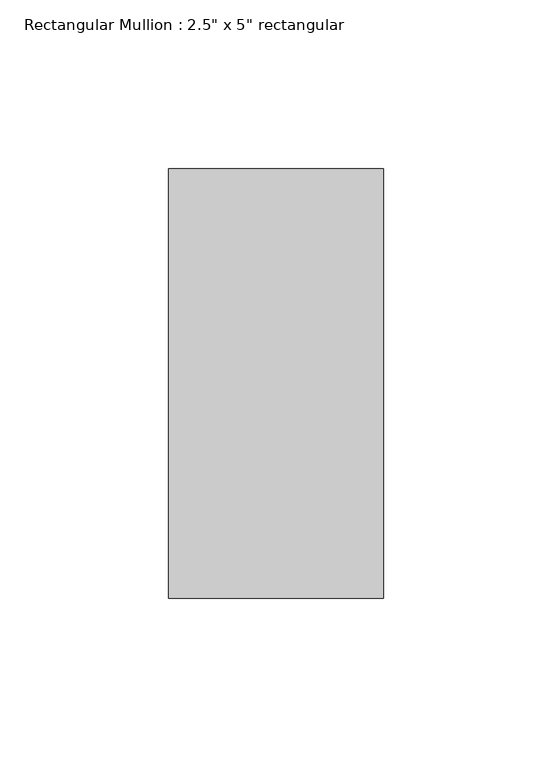
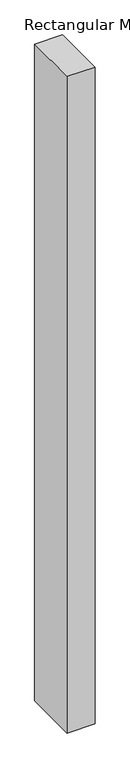
"""IFC4 building model written with IfcOpenShell, lengths in millimetres: member geometry."""

from ifc_helpers import new_model, si_unit, frame, origin, place, context, project, spatial, polyline, outline, extrude, source, transform, mapped, element, save


def member_6335abfa(model_context):
    return source(origin(), model_context, "Body", "SweptSolid", [
        extrude(outline(polyline([(0.0, 63.5), (0.0, -63.5), (-63.5, -63.5), (-63.5, 63.5), (0.0, 63.5)])), frame((0.0, 0.0, -1574.1253432), z_axis=(0.0, 0.0, 1.0), x_axis=(1.0, 0.0, 0.0)), (0.0, 0.0, 1.0), 1574.1253432),
    ])


if __name__ == "__main__":
    model = new_model("IFC4")
    model_context = context("Model", 3, world=origin())
    ifc_project = project(units=[si_unit("LENGTHUNIT", "METRE", prefix="MILLI")], contexts=[model_context])
    site = spatial("IfcSite", under=ifc_project)
    building = spatial("IfcBuilding", under=site)
    placement = place(None, origin())
    member_shape = member_6335abfa(model_context)
    element("IfcMember", 1, ObjectType="Rectangular Mullion : 2.5\" x 5\" rectangular", at=placement, inside=building, context=model_context, shape_type="MappedRepresentation", body=[
        mapped(member_shape, transform((0.0, 0.0, 0.0), x_axis=(1.0, 0.0, 0.0), y_axis=(0.0, 1.0, 0.0), z_axis=(0.0, 0.0, 1.0))),
    ])
    save(model, "model.ifc")

# Revit data of these elements
# Type "Rectangular Mullion : 2.5\" x 5\" rectangular"
#   built-in parameter 1007304 = 0.416667 (stored number, unit not read)
#   built-in parameter 1007301 = 0.104167 (stored number, unit not read)
#   built-in parameter 1007300 = 0.104167 (stored number, unit not read)
# Element 1 (IfcMember, "Rectangular Mullion : 2.5\" x 5\" rectangular")
#   Materials on its faces: "Aluminum"
# Materials
#   "Aluminum": class "Metal", colour RGB 247 247 247, transparency 0, Description = "Aluminum 6061", Cost = 0
